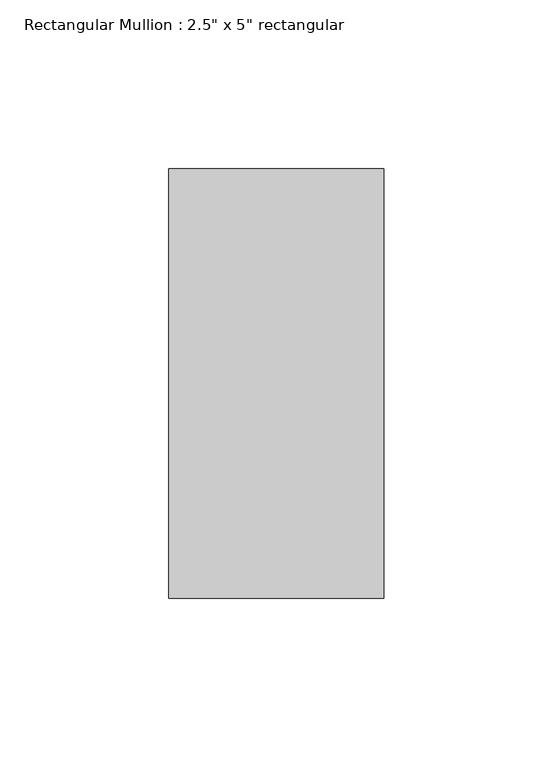
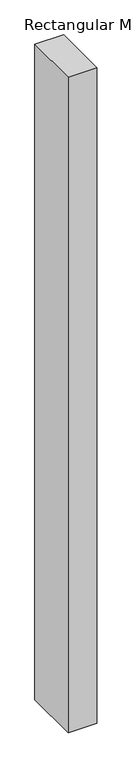
"""IFC4 building model written with IfcOpenShell, lengths in millimetres: member geometry."""

from ifc_helpers import new_model, si_unit, frame, origin, place, context, project, spatial, polyline, outline, extrude, source, transform, mapped, element, save


def member_2a2664cc(model_context):
    return source(origin(), model_context, "Body", "SweptSolid", [
        extrude(outline(polyline([(31.75, 63.5), (31.75, -63.5), (-31.75, -63.5), (-31.75, 63.5), (31.75, 63.5)])), frame((0.0, 0.0, -1533.754744), z_axis=(0.0, 0.0, 1.0), x_axis=(1.0, 0.0, 0.0)), (0.0, 0.0, 1.0), 1533.754744),
    ])


if __name__ == "__main__":
    model = new_model("IFC4")
    model_context = context("Model", 3, world=origin())
    ifc_project = project(units=[si_unit("LENGTHUNIT", "METRE", prefix="MILLI")], contexts=[model_context])
    site = spatial("IfcSite", under=ifc_project)
    building = spatial("IfcBuilding", under=site)
    placement = place(None, origin())
    member_shape = member_2a2664cc(model_context)
    element("IfcMember", 1, ObjectType="Rectangular Mullion : 2.5\" x 5\" rectangular", at=placement, inside=building, context=model_context, shape_type="MappedRepresentation", body=[
        mapped(member_shape, transform((0.0, 0.0, 0.0), x_axis=(1.0, 0.0, 0.0), y_axis=(0.0, 1.0, 0.0), z_axis=(0.0, 0.0, 1.0))),
    ])
    save(model, "model.ifc")

# Revit data of these elements
# Type "Rectangular Mullion : 2.5\" x 5\" rectangular"
#   built-in parameter 1007304 = 0.416667 (stored number, unit not read)
#   built-in parameter 1007301 = 0.104167 (stored number, unit not read)
#   built-in parameter 1007300 = 0.104167 (stored number, unit not read)
# Element 1 (IfcMember, "Rectangular Mullion : 2.5\" x 5\" rectangular")
#   Materials on its faces: "Aluminum"
# Materials
#   "Aluminum": class "Metal", colour RGB 247 247 247, transparency 0, Description = "Aluminum 6061", Cost = 0
